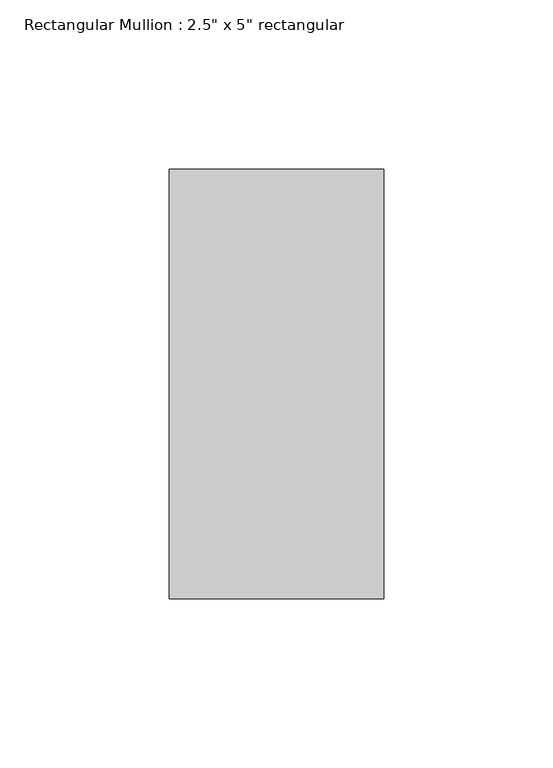
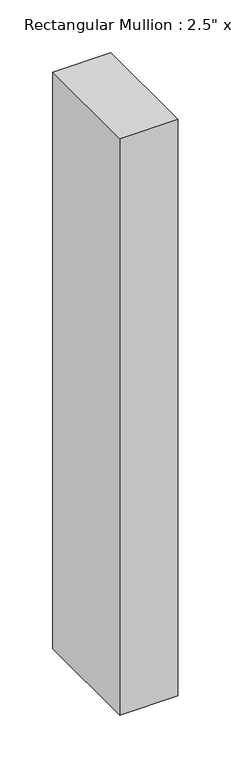
"""IFC4 building model written with IfcOpenShell, lengths in millimetres: member geometry."""

from ifc_helpers import new_model, si_unit, frame, origin, place, context, project, spatial, polyline, outline, extrude, source, transform, mapped, element, save


def member_c33c434a(model_context):
    return source(origin(), model_context, "Body", "SweptSolid", [
        extrude(outline(polyline([(0.0, 63.5), (0.0, -63.5), (-63.5, -63.5), (-63.5, 63.5), (0.0, 63.5)])), frame((0.0, 0.0, -666.75), z_axis=(0.0, 0.0, 1.0), x_axis=(1.0, 0.0, 0.0)), (0.0, 0.0, 1.0), 666.75),
    ])


if __name__ == "__main__":
    model = new_model("IFC4")
    model_context = context("Model", 3, world=origin())
    ifc_project = project(units=[si_unit("LENGTHUNIT", "METRE", prefix="MILLI")], contexts=[model_context])
    site = spatial("IfcSite", under=ifc_project)
    building = spatial("IfcBuilding", under=site)
    placement = place(None, origin())
    member_shape = member_c33c434a(model_context)
    element("IfcMember", 1, ObjectType="Rectangular Mullion : 2.5\" x 5\" rectangular", at=placement, inside=building, context=model_context, shape_type="MappedRepresentation", body=[
        mapped(member_shape, transform((0.0, 0.0, 0.0), x_axis=(1.0, 0.0, 0.0), y_axis=(0.0, 1.0, 0.0), z_axis=(0.0, 0.0, 1.0))),
    ])
    save(model, "model.ifc")

# Revit data of these elements
# Type "Rectangular Mullion : 2.5\" x 5\" rectangular"
#   built-in parameter 1007304 = 0.416667 (stored number, unit not read)
#   built-in parameter 1007301 = 0.104167 (stored number, unit not read)
#   built-in parameter 1007300 = 0.104167 (stored number, unit not read)
# Element 1 (IfcMember, "Rectangular Mullion : 2.5\" x 5\" rectangular")
#   Materials on its faces: "door black"
# Materials
#   "door black": class "Generic", colour RGB 120 120 120, transparency 0, Cost = 0
